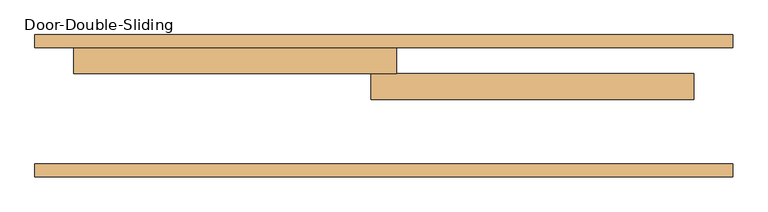
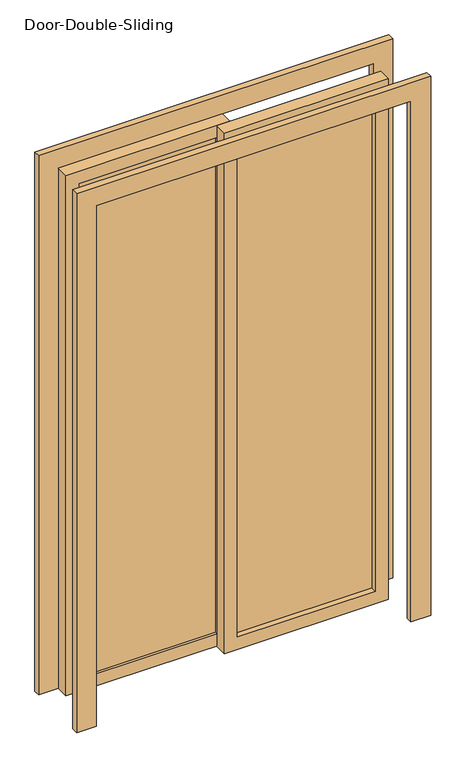
"""IFC4 building model written with IfcOpenShell, lengths in millimetres: door geometry, Door-Double-Sliding."""

from ifc_helpers import new_model, si_unit, frame, origin, place, context, project, spatial, polyline, outline, extrude, source, transform, mapped, element, save


def door_double_sliding_4436dcad(model_context):
    return source(origin(), model_context, "Body", "SweptSolid", [
        extrude(outline(polyline([(0.0, 685.8), (2209.8, 685.8), (2209.8, -685.8), (0.0, -685.8), (0.0, -609.6), (2133.6, -609.6), (2133.6, 609.6), (0.0, 609.6), (0.0, 685.8)])), frame((0.0, 241.3, 0.0), z_axis=(0.0, 1.0, 0.0), x_axis=(0.0, 0.0, 1.0)), (0.0, 0.0, 1.0), 25.4),
        extrude(outline(polyline([(0.0, -685.8), (0.0, -609.6), (2133.6, -609.6), (2133.6, 609.6), (0.0, 609.6), (0.0, 685.8), (2209.8, 685.8), (2209.8, -685.8), (0.0, -685.8)])), frame((0.0, -12.7, 0.0), z_axis=(0.0, 1.0, 0.0), x_axis=(0.0, 0.0, 1.0)), (0.0, 0.0, 1.0), 25.4),
        extrude(outline(polyline([(2133.6, 25.4), (2133.6, -609.6), (0.0, -609.6), (0.0, 25.4), (2133.6, 25.4)]), holes=[polyline([(2082.8, -25.4), (50.8, -25.4), (50.8, -558.8), (2082.8, -558.8), (2082.8, -25.4)])]), frame((0.0, 190.5, 0.0), z_axis=(0.0, 1.0, 0.0), x_axis=(0.0, 0.0, 1.0)), (0.0, 0.0, 1.0), 50.8),
        extrude(outline(polyline([(2133.6, -25.4), (0.0, -25.4), (0.0, 609.6), (2133.6, 609.6), (2133.6, -25.4)]), holes=[polyline([(2082.8, 25.4), (2082.8, 558.8), (50.8, 558.8), (50.8, 25.4), (2082.8, 25.4)])]), frame((0.0, 139.7, 0.0), z_axis=(0.0, 1.0, 0.0), x_axis=(0.0, 0.0, 1.0)), (0.0, 0.0, 1.0), 50.8),
        extrude(outline(polyline([(-25.4, 200.025), (-558.8, 200.025), (-558.8, 206.375), (-25.4, 206.375), (-25.4, 200.025)])), frame((0.0, 0.0, 50.8), z_axis=(0.0, 0.0, 1.0), x_axis=(1.0, 0.0, 0.0)), (0.0, 0.0, 1.0), 2032.0),
        extrude(outline(polyline([(25.4, 168.275), (558.8, 168.275), (558.8, 161.925), (25.4, 161.925), (25.4, 168.275)])), frame((0.0, 0.0, 50.8), z_axis=(0.0, 0.0, 1.0), x_axis=(1.0, 0.0, 0.0)), (0.0, 0.0, 1.0), 2032.0),
    ])


if __name__ == "__main__":
    model = new_model("IFC4")
    model_context = context("Model", 3, world=origin())
    ifc_project = project(units=[si_unit("LENGTHUNIT", "METRE", prefix="MILLI")], contexts=[model_context])
    site = spatial("IfcSite", under=ifc_project)
    building = spatial("IfcBuilding", under=site)
    placement = place(None, origin())
    door_double_sliding_shape = door_double_sliding_4436dcad(model_context)
    element("IfcDoor", 1, ObjectType="Door-Double-Sliding", at=placement, inside=building, context=model_context, shape_type="MappedRepresentation", body=[
        mapped(door_double_sliding_shape, transform((0.0, 0.0, 0.0), x_axis=(1.0, 0.0, 0.0), y_axis=(0.0, 1.0, 0.0), z_axis=(0.0, 0.0, 1.0))),
    ])
    save(model, "model.ifc")

# Revit data of these elements
# Type "Door-Double-Sliding"
#   Type Mark = "14"
#   Construction Type Id = "opn-d45"
#   Assembly Code = "C1020"
#   Analytic Construction = "Wood frame, double glass door "
#   Thickness = 0' - 2"
#   Thermal Resistance (R) = 1.8150 (h·ft²·°F)/BTU
#   Heat Transfer Coefficient (U) = 0.5510 BTU/(h·ft²·°F)
#   Height = 7' - 0"
#   Rail Width = 0' - 2"
#   Stiles = 0' - 2"
#   Trim Projection Ext = 0' - 1"
#   Trim Projection Int = 0' - 1"
#   Trim Width = 0' - 3"
#   Width = 4' - 0"
#   Define Thermal Properties by = 1
#   Glazing = Glass
#   Panel Material = Wood - Birch - Solid Stained Light Low Gloss
#   Trim Material = Paint - Sienna
#   Visual Light Transmittance = 0
#   Solar Heat Gain Coefficient = 0
#   Function = (empty or 0)
#   Wall Closure = (empty or 0)
# Element 1 (IfcDoor, "Door-Double-Sliding")
#   Materials on its faces: "Paint - Sienna", "Wood - Birch - Solid Stained Light Low Gloss", "Glass"
# Materials
#   "Glass": class "Glass", colour RGB 0 128 192, transparency 0.75, Description = "Soda Lime Glass", Cost = 0
#   "Wood - Birch - Solid Stained Light Low Gloss": class "Wood", colour RGB 210 159 95, transparency 0, Cost = 0
#   "Paint - Sienna": colour RGB 118 70 51, transparency 0, Cost = 0
